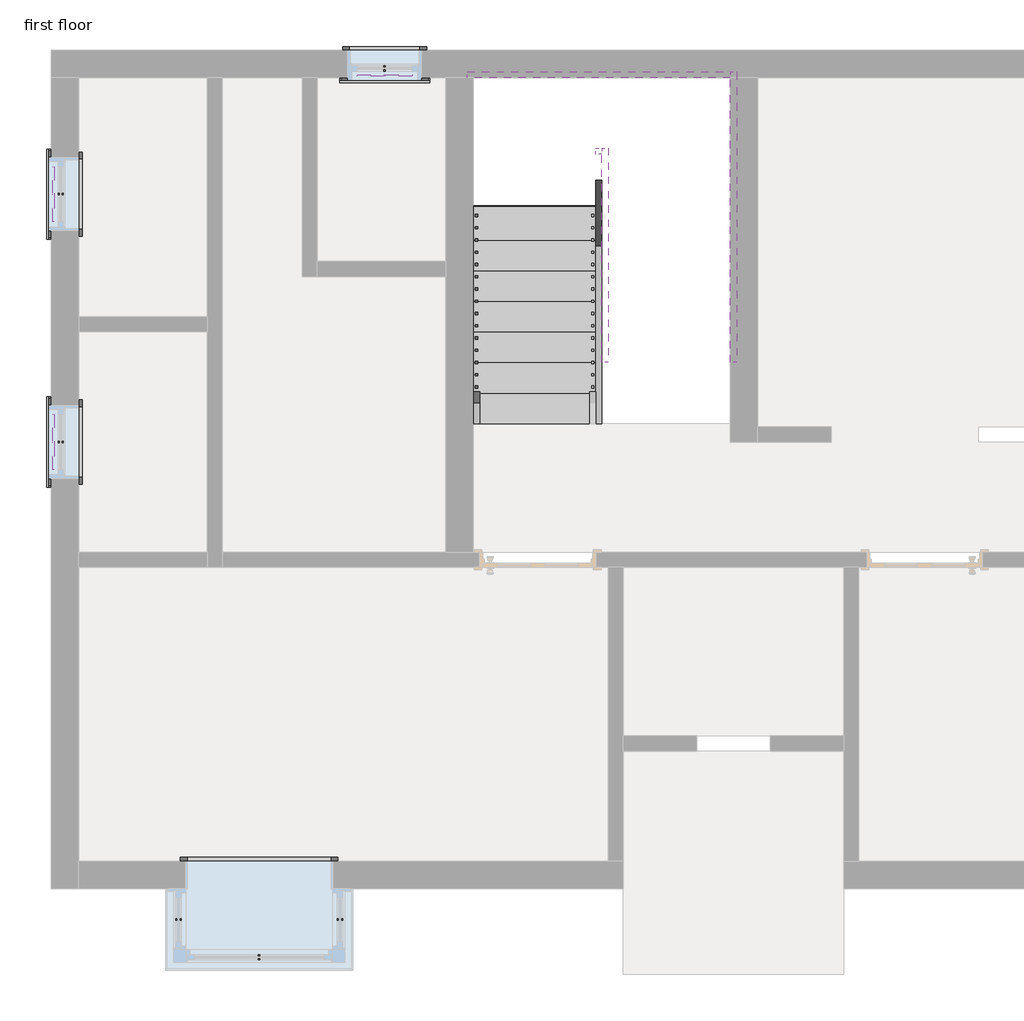
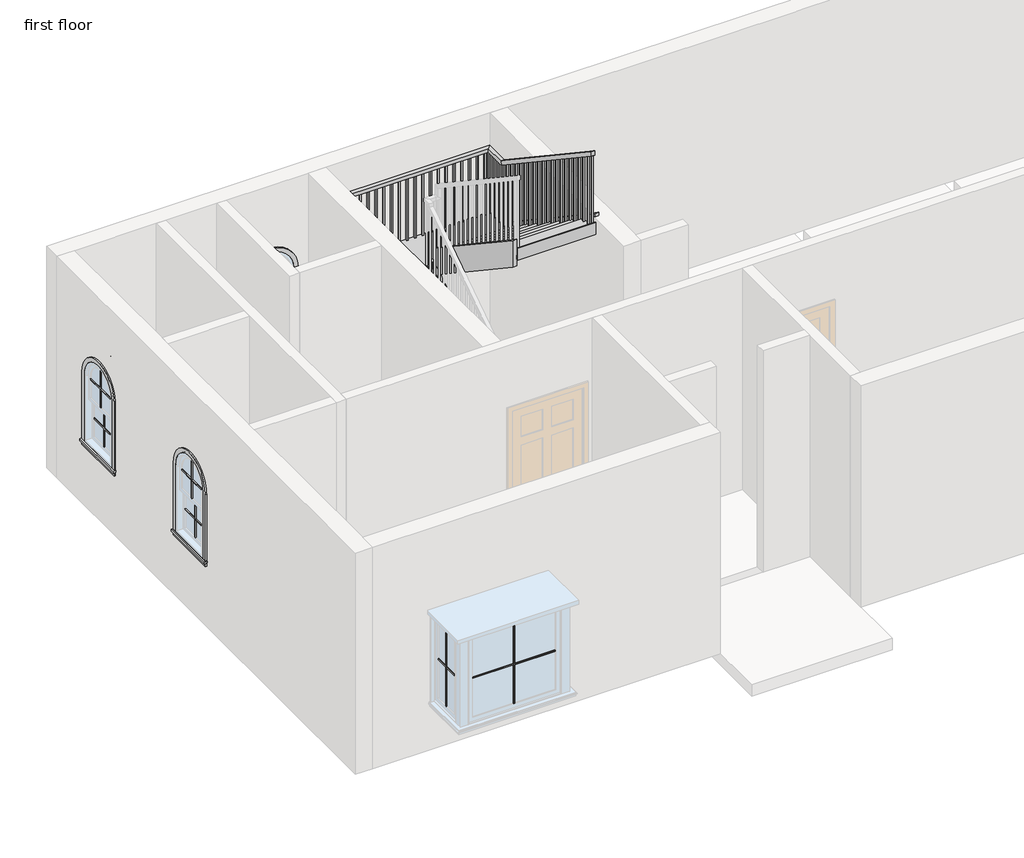
# One storey, part 3 of 3: 16 proxies, 6 members, 1 railing, 1 stair flight.
"""IFC4 building model written with IfcOpenShell, lengths in millimetres."""

from ifc_helpers import new_model, si_unit, frame, origin, place, context, project, spatial, polyline, outline, extrude, faceted_brep, transform, mapped, element, save
from components import muntin_pattern_2x2_muntin_pattern_2x2_3440c8d2, muntin_pattern_2x2_muntin_pattern_2x2_8235f178, muntin_pattern_2x2_muntin_pattern_2x2_f03ab90d, trim_window_exterior_arch_hung_with_sill_ae9dfc94, trim_window_interior_arch_hung_picture_frame_76300bdb, trim_window_interior_flat_picture_frame_ace0ae79, stair_flight_5c93b7ad

model = new_model("IFC4")

# Units and contexts
model_context = context("Model", 3, world=origin())
ifc_project = project(units=[si_unit("LENGTHUNIT", "METRE", prefix="MILLI")], contexts=[model_context])

# Site, building, storey
site = spatial("IfcSite", under=ifc_project)
building = spatial("IfcBuilding", under=site)
storey = spatial("IfcBuildingStorey", under=building, Name="first floor", Elevation=3352.8)

# Proxies
placement = place(None, origin())
muntin_pattern_2x2_muntin_pattern_2x2_shape = muntin_pattern_2x2_muntin_pattern_2x2_3440c8d2(model_context)
element("IfcBuildingElementProxy", 1, Name="Muntin Pattern_2x2 : Muntin Pattern_2x2", ObjectType="Muntin Pattern_2x2 : Muntin Pattern_2x2", at=placement, inside=storey, context=model_context, shape_type="MappedRepresentation", body=[
    mapped(muntin_pattern_2x2_muntin_pattern_2x2_shape, transform((-13144.1422301, -1499.4302427, 4899.025), x_axis=(0.0, 1.0, 0.0), y_axis=(-1.0, 0.0, 0.0), z_axis=(0.0, 0.0, 1.0))),
])
element("IfcBuildingElementProxy", 2, Name="Muntin Pattern_2x2 : Muntin Pattern_2x2", ObjectType="Muntin Pattern_2x2 : Muntin Pattern_2x2", at=placement, inside=storey, context=model_context, shape_type="MappedRepresentation", body=[
    mapped(muntin_pattern_2x2_muntin_pattern_2x2_shape, transform((-13099.6922301, -1499.4302427, 4343.4), x_axis=(0.0, 1.0, 0.0), y_axis=(-1.0, 0.0, 0.0), z_axis=(0.0, 0.0, 1.0))),
])
element("IfcBuildingElementProxy", 3, Name="Muntin Pattern_2x2 : Muntin Pattern_2x2", ObjectType="Muntin Pattern_2x2 : Muntin Pattern_2x2", at=placement, inside=storey, context=model_context, shape_type="MappedRepresentation", body=[
    mapped(muntin_pattern_2x2_muntin_pattern_2x2_shape, transform((-13144.1422301, -3556.8302427, 4899.025), x_axis=(0.0, 1.0, 0.0), y_axis=(-1.0, 0.0, 0.0), z_axis=(0.0, 0.0, 1.0))),
])
element("IfcBuildingElementProxy", 4, Name="Muntin Pattern_2x2 : Muntin Pattern_2x2", ObjectType="Muntin Pattern_2x2 : Muntin Pattern_2x2", at=placement, inside=storey, context=model_context, shape_type="MappedRepresentation", body=[
    mapped(muntin_pattern_2x2_muntin_pattern_2x2_shape, transform((-13099.6922301, -3556.8302427, 4343.4), x_axis=(0.0, 1.0, 0.0), y_axis=(-1.0, 0.0, 0.0), z_axis=(0.0, 0.0, 1.0))),
])
element("IfcBuildingElementProxy", 5, Name="Muntin Pattern_2x2 : Muntin Pattern_2x2", ObjectType="Muntin Pattern_2x2 : Muntin Pattern_2x2", at=placement, inside=storey, context=model_context, shape_type="MappedRepresentation", body=[
    mapped(muntin_pattern_2x2_muntin_pattern_2x2_shape, transform((-10410.4672301, -499.3052427, 4899.025), x_axis=(-1.0, 0.0, 0.0), y_axis=(0.0, -1.0, 0.0), z_axis=(0.0, 0.0, 1.0))),
])
element("IfcBuildingElementProxy", 6, Name="Muntin Pattern_2x2 : Muntin Pattern_2x2", ObjectType="Muntin Pattern_2x2 : Muntin Pattern_2x2", at=placement, inside=storey, context=model_context, shape_type="MappedRepresentation", body=[
    mapped(muntin_pattern_2x2_muntin_pattern_2x2_shape, transform((-10410.4672301, -454.8552427, 4343.4), x_axis=(-1.0, 0.0, 0.0), y_axis=(0.0, -1.0, 0.0), z_axis=(0.0, 0.0, 1.0))),
])
muntin_pattern_2x2_muntin_pattern_2x2_2_shape = muntin_pattern_2x2_muntin_pattern_2x2_8235f178(model_context)
element("IfcBuildingElementProxy", 7, Name="Muntin Pattern_2x2 : Muntin Pattern_2x2", ObjectType="Muntin Pattern_2x2 : Muntin Pattern_2x2", at=placement, inside=storey, context=model_context, shape_type="MappedRepresentation", body=[
    mapped(muntin_pattern_2x2_muntin_pattern_2x2_2_shape, transform((-11451.8672301, -7833.5552427, 4083.05), x_axis=(-1.0, 0.0, 0.0), y_axis=(0.0, -1.0, 0.0), z_axis=(0.0, 0.0, 1.0))),
])
muntin_pattern_2x2_muntin_pattern_2x2_3_shape = muntin_pattern_2x2_muntin_pattern_2x2_f03ab90d(model_context)
element("IfcBuildingElementProxy", 8, Name="Muntin Pattern_2x2 : Muntin Pattern_2x2", ObjectType="Muntin Pattern_2x2 : Muntin Pattern_2x2", at=placement, inside=storey, context=model_context, shape_type="MappedRepresentation", body=[
    mapped(muntin_pattern_2x2_muntin_pattern_2x2_3_shape, transform((-10781.9422301, -7519.2302427, 4083.05), x_axis=(0.0, 1.0, 0.0), y_axis=(-1.0, 0.0, 0.0), z_axis=(0.0, 0.0, 1.0))),
])
element("IfcBuildingElementProxy", 9, Name="Muntin Pattern_2x2 : Muntin Pattern_2x2", ObjectType="Muntin Pattern_2x2 : Muntin Pattern_2x2", at=placement, inside=storey, context=model_context, shape_type="MappedRepresentation", body=[
    mapped(muntin_pattern_2x2_muntin_pattern_2x2_3_shape, transform((-12121.7922301, -7519.2302427, 4083.05), x_axis=(0.0, -1.0, 0.0), y_axis=(1.0, 0.0, 0.0), z_axis=(0.0, 0.0, 1.0))),
])
trim_window_exterior_arch_hung_with_sill_shape = trim_window_exterior_arch_hung_with_sill_ae9dfc94(model_context)
element("IfcBuildingElementProxy", 10, Name="Trim-Window-Exterior-Arch-Hung : with Sill", ObjectType="Trim-Window-Exterior-Arch-Hung : with Sill", at=placement, inside=storey, context=model_context, shape_type="MappedRepresentation", body=[
    mapped(trim_window_exterior_arch_hung_with_sill_shape, transform((-13179.0672301, -1499.4302427, 5486.4), x_axis=(0.0, -1.0, 0.0), y_axis=(0.0, 0.0, 1.0), z_axis=(-1.0, 0.0, 0.0))),
])
element("IfcBuildingElementProxy", 11, Name="Trim-Window-Exterior-Arch-Hung : with Sill", ObjectType="Trim-Window-Exterior-Arch-Hung : with Sill", at=placement, inside=storey, context=model_context, shape_type="MappedRepresentation", body=[
    mapped(trim_window_exterior_arch_hung_with_sill_shape, transform((-13179.0672301, -3556.8302427, 5486.4), x_axis=(0.0, -1.0, 0.0), y_axis=(0.0, 0.0, 1.0), z_axis=(-1.0, 0.0, 0.0))),
])
element("IfcBuildingElementProxy", 12, Name="Trim-Window-Exterior-Arch-Hung : with Sill", ObjectType="Trim-Window-Exterior-Arch-Hung : with Sill", at=placement, inside=storey, context=model_context, shape_type="MappedRepresentation", body=[
    mapped(trim_window_exterior_arch_hung_with_sill_shape, transform((-10410.4672301, -534.2302427, 5486.4), x_axis=(1.0, 0.0, 0.0), y_axis=(0.0, 0.0, 1.0), z_axis=(0.0, -1.0, 0.0))),
])
trim_window_interior_arch_hung_picture_frame_shape = trim_window_interior_arch_hung_picture_frame_76300bdb(model_context)
element("IfcBuildingElementProxy", 13, Name="Trim-Window-Interior-Arch-Hung : Picture Frame", ObjectType="Trim-Window-Interior-Arch-Hung : Picture Frame", at=placement, inside=storey, context=model_context, shape_type="MappedRepresentation", body=[
    mapped(trim_window_interior_arch_hung_picture_frame_shape, transform((-12950.4672301, -1499.4302427, 5486.4), x_axis=(0.0, 1.0, 0.0), y_axis=(0.0, 0.0, 1.0), z_axis=(1.0, 0.0, 0.0))),
])
element("IfcBuildingElementProxy", 14, Name="Trim-Window-Interior-Arch-Hung : Picture Frame", ObjectType="Trim-Window-Interior-Arch-Hung : Picture Frame", at=placement, inside=storey, context=model_context, shape_type="MappedRepresentation", body=[
    mapped(trim_window_interior_arch_hung_picture_frame_shape, transform((-12950.4672301, -3556.8302427, 5486.4), x_axis=(0.0, 1.0, 0.0), y_axis=(0.0, 0.0, 1.0), z_axis=(1.0, 0.0, 0.0))),
])
element("IfcBuildingElementProxy", 15, Name="Trim-Window-Interior-Arch-Hung : Picture Frame", ObjectType="Trim-Window-Interior-Arch-Hung : Picture Frame", at=placement, inside=storey, context=model_context, shape_type="MappedRepresentation", body=[
    mapped(trim_window_interior_arch_hung_picture_frame_shape, transform((-10410.4672301, -305.6302427, 5486.4), x_axis=(-1.0, 0.0, 0.0), y_axis=(0.0, 0.0, 1.0), z_axis=(0.0, 1.0, 0.0))),
])
trim_window_interior_flat_picture_frame_shape = trim_window_interior_flat_picture_frame_ace0ae79(model_context)
element("IfcBuildingElementProxy", 16, Name="Trim-Window-Interior-Flat : Picture Frame", ObjectType="Trim-Window-Interior-Flat : Picture Frame", at=placement, inside=storey, context=model_context, shape_type="MappedRepresentation", body=[
    mapped(trim_window_interior_flat_picture_frame_shape, transform((-11451.8672301, -7036.6302427, 5232.4), x_axis=(-1.0, 0.0, 0.0), y_axis=(0.0, 0.0, 1.0), z_axis=(0.0, 1.0, 0.0))),
])

# Members
element("IfcMember", 17, ObjectType="Stringer - 2\" Width", at=placement, inside=storey, context=model_context, shape_type="SweptSolid", body=[
    extrude(outline(polyline([(-3404.4302427, 3352.8), (-3404.4302427, 3570.8398409), (-1077.1900041, 5122.3333333), (-534.2302427, 5122.3333333), (-534.2302427, 5117.982498), (-3182.0039897, 3352.8), (-3404.4302427, 3352.8)])), frame((-9724.6672301, 0.0, 0.0), z_axis=(1.0, 0.0, 0.0), x_axis=(0.0, 1.0, 0.0)), (0.0, 0.0, 1.0), 50.8),
])
element("IfcMember", 18, ObjectType="Stringer - 2\" Width", at=placement, inside=storey, context=model_context, shape_type="SweptSolid", body=[
    extrude(outline(polyline([(-9724.6672301, -534.2302427), (-9724.6672301, -483.4302427), (-7540.2672301, -483.4302427), (-7540.2672301, -534.2302427), (-9724.6672301, -534.2302427)])), frame((0.0, 0.0, 4817.5333333), z_axis=(0.0, 0.0, 1.0), x_axis=(1.0, 0.0, 0.0)), (0.0, 0.0, 1.0), 304.8),
])
element("IfcMember", 19, ObjectType="Stringer - 2\" Width", at=placement, inside=storey, context=model_context, shape_type="SweptSolid", body=[
    extrude(outline(polyline([(-483.4302427, 4840.8398409), (-483.4302427, 4817.5333333), (-997.9564957, 4817.5333333), (-2896.4302427, 6083.182498), (-2896.4302427, 6449.5065076), (-483.4302427, 4840.8398409)])), frame((-7540.2672301, 0.0, 0.0), z_axis=(1.0, 0.0, 0.0), x_axis=(0.0, 1.0, 0.0)), (0.0, 0.0, 1.0), 50.8),
])
element("IfcMember", 20, ObjectType="Stringer - 2\" Width", at=placement, inside=storey, context=model_context, shape_type="SweptSolid", body=[
    extrude(outline(polyline([(-3404.4302427, 3352.8), (-3404.4302427, 3570.8398409), (-1169.2302427, 5060.9731743), (-1169.2302427, 4694.6491647), (-3182.0039897, 3352.8), (-3404.4302427, 3352.8)])), frame((-8657.8672301, 0.0, 0.0), z_axis=(1.0, 0.0, 0.0), x_axis=(0.0, 1.0, 0.0)), (0.0, 0.0, 1.0), 50.8),
])
element("IfcMember", 21, ObjectType="Stringer - 2\" Width", at=placement, inside=storey, context=model_context, shape_type="SweptSolid", body=[
    extrude(outline(polyline([(-8657.8672301, -1169.2302427), (-8657.8672301, -1118.4302427), (-8607.0672301, -1118.4302427), (-8607.0672301, -1169.2302427), (-8657.8672301, -1169.2302427)])), frame((0.0, 0.0, 4817.5333333), z_axis=(0.0, 0.0, 1.0), x_axis=(1.0, 0.0, 0.0)), (0.0, 0.0, 1.0), 304.8),
])
element("IfcMember", 22, ObjectType="Stringer - 2\" Width", at=placement, inside=storey, context=model_context, shape_type="SweptSolid", body=[
    extrude(outline(polyline([(-1118.4302427, 5264.1731743), (-1118.4302427, 4897.8491647), (-2896.4302427, 6083.182498), (-2896.4302427, 6449.5065076), (-1118.4302427, 5264.1731743)])), frame((-8607.0672301, 0.0, 0.0), z_axis=(1.0, 0.0, 0.0), x_axis=(0.0, 1.0, 0.0)), (0.0, 0.0, 1.0), 50.8),
])

# Railing
element("IfcRailing", 23, ObjectType="Handrail - Rectangular", at=placement, inside=storey, context=model_context, shape_type="SolidModel", body=[
    faceted_brep([(-9673.8672301, -3404.4302427, 4436.5333333), (-9673.8672301, -3404.4302427, 4375.4793317), (-9623.0672301, -3404.4302427, 4375.4793317), (-9623.0672301, -3404.4302427, 4436.5333333), (-9673.8672301, -1118.4302427, 5960.5333333), (-9673.8672301, -1103.0492403, 5909.7333333), (-9623.0672301, -1103.0492403, 5909.7333333), (-9623.0672301, -1118.4302427, 5960.5333333), (-9673.8672301, -534.2302427, 5960.5333333), (-9673.8672301, -534.2302427, 5909.7333333), (-9623.0672301, -585.0302427, 5909.7333333), (-9623.0672301, -585.0302427, 5960.5333333), (-7540.2672301, -534.2302427, 5960.5333333), (-7540.2672301, -534.2302427, 5909.7333333), (-7591.0672301, -585.0302427, 5909.7333333), (-7591.0672301, -585.0302427, 5960.5333333), (-7540.2672301, -864.4302427, 5960.5333333), (-7540.2672301, -879.8112451, 5909.7333333), (-7591.0672301, -879.8112451, 5909.7333333), (-7591.0672301, -864.4302427, 5960.5333333), (-7540.2672301, -2896.4302427, 7315.2), (-7591.0672301, -2896.4302427, 7315.2), (-7591.0672301, -2896.4302427, 7254.1459984), (-7540.2672301, -2896.4302427, 7254.1459984)], [[[0, 1, 2, 3]], [[1, 0, 4, 5]], [[2, 1, 5, 6]], [[3, 2, 6, 7]], [[0, 3, 7, 4]], [[5, 4, 8, 9]], [[6, 5, 9, 10]], [[7, 6, 10, 11]], [[4, 7, 11, 8]], [[9, 8, 12, 13]], [[10, 9, 13, 14]], [[11, 10, 14, 15]], [[8, 11, 15, 12]], [[13, 12, 16, 17]], [[14, 13, 17, 18]], [[15, 14, 18, 19]], [[12, 15, 19, 16]], [[20, 21, 22, 23]], [[17, 16, 20, 23]], [[18, 17, 23, 22]], [[19, 18, 22, 21]], [[16, 19, 21, 20]]]),
    extrude(outline(polyline([(-2785.3052427, 7180.0626651), (-2785.3052427, 6231.4666667), (-2804.3552427, 6231.4666667), (-2804.3552427, 7192.7626651), (-2785.3052427, 7180.0626651)])), frame((-7575.1922301, 0.0, 0.0), z_axis=(1.0, 0.0, 0.0), x_axis=(0.0, 1.0, 0.0)), (0.0, 0.0, 1.0), 19.05),
    extrude(outline(polyline([(-2683.7052427, 7112.3293317), (-2683.7052427, 6231.4666667), (-2702.7552427, 6231.4666667), (-2702.7552427, 7125.0293317), (-2683.7052427, 7112.3293317)])), frame((-7575.1922301, 0.0, 0.0), z_axis=(1.0, 0.0, 0.0), x_axis=(0.0, 1.0, 0.0)), (0.0, 0.0, 1.0), 19.05),
    extrude(outline(polyline([(-2582.1052427, 7044.5959984), (-2582.1052427, 6062.1333333), (-2601.1552427, 6062.1333333), (-2601.1552427, 7057.2959984), (-2582.1052427, 7044.5959984)])), frame((-7575.1922301, 0.0, 0.0), z_axis=(1.0, 0.0, 0.0), x_axis=(0.0, 1.0, 0.0)), (0.0, 0.0, 1.0), 19.05),
    extrude(outline(polyline([(-2480.5052427, 6976.8626651), (-2480.5052427, 6062.1333333), (-2499.5552427, 6062.1333333), (-2499.5552427, 6989.5626651), (-2480.5052427, 6976.8626651)])), frame((-7575.1922301, 0.0, 0.0), z_axis=(1.0, 0.0, 0.0), x_axis=(0.0, 1.0, 0.0)), (0.0, 0.0, 1.0), 19.05),
    extrude(outline(polyline([(-2378.9052427, 6909.1293317), (-2378.9052427, 6062.1333333), (-2397.9552427, 6062.1333333), (-2397.9552427, 6921.8293317), (-2378.9052427, 6909.1293317)])), frame((-7575.1922301, 0.0, 0.0), z_axis=(1.0, 0.0, 0.0), x_axis=(0.0, 1.0, 0.0)), (0.0, 0.0, 1.0), 19.05),
    extrude(outline(polyline([(-2277.3052427, 6841.3959984), (-2277.3052427, 5892.8), (-2296.3552427, 5892.8), (-2296.3552427, 6854.0959984), (-2277.3052427, 6841.3959984)])), frame((-7575.1922301, 0.0, 0.0), z_axis=(1.0, 0.0, 0.0), x_axis=(0.0, 1.0, 0.0)), (0.0, 0.0, 1.0), 19.05),
    extrude(outline(polyline([(-2175.7052427, 6773.6626651), (-2175.7052427, 5892.8), (-2194.7552427, 5892.8), (-2194.7552427, 6786.3626651), (-2175.7052427, 6773.6626651)])), frame((-7575.1922301, 0.0, 0.0), z_axis=(1.0, 0.0, 0.0), x_axis=(0.0, 1.0, 0.0)), (0.0, 0.0, 1.0), 19.05),
    extrude(outline(polyline([(-2074.1052427, 6705.9293317), (-2074.1052427, 5723.4666667), (-2093.1552427, 5723.4666667), (-2093.1552427, 6718.6293317), (-2074.1052427, 6705.9293317)])), frame((-7575.1922301, 0.0, 0.0), z_axis=(1.0, 0.0, 0.0), x_axis=(0.0, 1.0, 0.0)), (0.0, 0.0, 1.0), 19.05),
    extrude(outline(polyline([(-1972.5052427, 6638.1959984), (-1972.5052427, 5723.4666667), (-1991.5552427, 5723.4666667), (-1991.5552427, 6650.8959984), (-1972.5052427, 6638.1959984)])), frame((-7575.1922301, 0.0, 0.0), z_axis=(1.0, 0.0, 0.0), x_axis=(0.0, 1.0, 0.0)), (0.0, 0.0, 1.0), 19.05),
    extrude(outline(polyline([(-1870.9052427, 6570.4626651), (-1870.9052427, 5723.4666667), (-1889.9552427, 5723.4666667), (-1889.9552427, 6583.1626651), (-1870.9052427, 6570.4626651)])), frame((-7575.1922301, 0.0, 0.0), z_axis=(1.0, 0.0, 0.0), x_axis=(0.0, 1.0, 0.0)), (0.0, 0.0, 1.0), 19.05),
    extrude(outline(polyline([(-1769.3052427, 6502.7293317), (-1769.3052427, 5554.1333333), (-1788.3552427, 5554.1333333), (-1788.3552427, 6515.4293317), (-1769.3052427, 6502.7293317)])), frame((-7575.1922301, 0.0, 0.0), z_axis=(1.0, 0.0, 0.0), x_axis=(0.0, 1.0, 0.0)), (0.0, 0.0, 1.0), 19.05),
    extrude(outline(polyline([(-1667.7052427, 6434.9959984), (-1667.7052427, 5554.1333333), (-1686.7552427, 5554.1333333), (-1686.7552427, 6447.6959984), (-1667.7052427, 6434.9959984)])), frame((-7575.1922301, 0.0, 0.0), z_axis=(1.0, 0.0, 0.0), x_axis=(0.0, 1.0, 0.0)), (0.0, 0.0, 1.0), 19.05),
    extrude(outline(polyline([(-1566.1052427, 6367.2626651), (-1566.1052427, 5384.8), (-1585.1552427, 5384.8), (-1585.1552427, 6379.9626651), (-1566.1052427, 6367.2626651)])), frame((-7575.1922301, 0.0, 0.0), z_axis=(1.0, 0.0, 0.0), x_axis=(0.0, 1.0, 0.0)), (0.0, 0.0, 1.0), 19.05),
    extrude(outline(polyline([(-1464.5052427, 6299.5293317), (-1464.5052427, 5384.8), (-1483.5552427, 5384.8), (-1483.5552427, 6312.2293317), (-1464.5052427, 6299.5293317)])), frame((-7575.1922301, 0.0, 0.0), z_axis=(1.0, 0.0, 0.0), x_axis=(0.0, 1.0, 0.0)), (0.0, 0.0, 1.0), 19.05),
    extrude(outline(polyline([(-1362.9052427, 6231.7959984), (-1362.9052427, 5384.8), (-1381.9552427, 5384.8), (-1381.9552427, 6244.4959984), (-1362.9052427, 6231.7959984)])), frame((-7575.1922301, 0.0, 0.0), z_axis=(1.0, 0.0, 0.0), x_axis=(0.0, 1.0, 0.0)), (0.0, 0.0, 1.0), 19.05),
    extrude(outline(polyline([(-1261.3052427, 6164.0626651), (-1261.3052427, 5215.4666667), (-1280.3552427, 5215.4666667), (-1280.3552427, 6176.7626651), (-1261.3052427, 6164.0626651)])), frame((-7575.1922301, 0.0, 0.0), z_axis=(1.0, 0.0, 0.0), x_axis=(0.0, 1.0, 0.0)), (0.0, 0.0, 1.0), 19.05),
    extrude(outline(polyline([(-1159.7052427, 6096.3293317), (-1159.7052427, 5215.4666667), (-1178.7552427, 5215.4666667), (-1178.7552427, 6109.0293317), (-1159.7052427, 6096.3293317)])), frame((-7575.1922301, 0.0, 0.0), z_axis=(1.0, 0.0, 0.0), x_axis=(0.0, 1.0, 0.0)), (0.0, 0.0, 1.0), 19.05),
    extrude(outline(polyline([(-1058.1052427, 6028.5959984), (-1058.1052427, 5046.1333333), (-1077.1552427, 5046.1333333), (-1077.1552427, 6041.2959984), (-1058.1052427, 6028.5959984)])), frame((-7575.1922301, 0.0, 0.0), z_axis=(1.0, 0.0, 0.0), x_axis=(0.0, 1.0, 0.0)), (0.0, 0.0, 1.0), 19.05),
    extrude(outline(polyline([(-956.5052427, 5960.8626651), (-956.5052427, 5046.1333333), (-975.5552427, 5046.1333333), (-975.5552427, 5973.5626651), (-956.5052427, 5960.8626651)])), frame((-7575.1922301, 0.0, 0.0), z_axis=(1.0, 0.0, 0.0), x_axis=(0.0, 1.0, 0.0)), (0.0, 0.0, 1.0), 19.05),
    extrude(outline(polyline([(-7556.1422301, -854.9052427), (-7556.1422301, -873.9552427), (-7575.1922301, -873.9552427), (-7575.1922301, -854.9052427), (-7556.1422301, -854.9052427)])), frame((0.0, 0.0, 5046.1333333), z_axis=(0.0, 0.0, 1.0), x_axis=(1.0, 0.0, 0.0)), (0.0, 0.0, 1.0), 863.6),
    extrude(outline(polyline([(-7556.1422301, -753.3052427), (-7556.1422301, -772.3552427), (-7575.1922301, -772.3552427), (-7575.1922301, -753.3052427), (-7556.1422301, -753.3052427)])), frame((0.0, 0.0, 5046.1333333), z_axis=(0.0, 0.0, 1.0), x_axis=(1.0, 0.0, 0.0)), (0.0, 0.0, 1.0), 863.6),
    extrude(outline(polyline([(-7556.1422301, -651.7052427), (-7556.1422301, -670.7552427), (-7575.1922301, -670.7552427), (-7575.1922301, -651.7052427), (-7556.1422301, -651.7052427)])), frame((0.0, 0.0, 5046.1333333), z_axis=(0.0, 0.0, 1.0), x_axis=(1.0, 0.0, 0.0)), (0.0, 0.0, 1.0), 863.6),
    extrude(outline(polyline([(-7625.9922301, -550.1052427), (-7606.9422301, -550.1052427), (-7606.9422301, -569.1552427), (-7625.9922301, -569.1552427), (-7625.9922301, -550.1052427)])), frame((0.0, 0.0, 5046.1333333), z_axis=(0.0, 0.0, 1.0), x_axis=(1.0, 0.0, 0.0)), (0.0, 0.0, 1.0), 863.6),
    extrude(outline(polyline([(-7727.5922301, -550.1052427), (-7708.5422301, -550.1052427), (-7708.5422301, -569.1552427), (-7727.5922301, -569.1552427), (-7727.5922301, -550.1052427)])), frame((0.0, 0.0, 5046.1333333), z_axis=(0.0, 0.0, 1.0), x_axis=(1.0, 0.0, 0.0)), (0.0, 0.0, 1.0), 863.6),
    extrude(outline(polyline([(-7829.1922301, -550.1052427), (-7810.1422301, -550.1052427), (-7810.1422301, -569.1552427), (-7829.1922301, -569.1552427), (-7829.1922301, -550.1052427)])), frame((0.0, 0.0, 5046.1333333), z_axis=(0.0, 0.0, 1.0), x_axis=(1.0, 0.0, 0.0)), (0.0, 0.0, 1.0), 863.6),
    extrude(outline(polyline([(-7930.7922301, -550.1052427), (-7911.7422301, -550.1052427), (-7911.7422301, -569.1552427), (-7930.7922301, -569.1552427), (-7930.7922301, -550.1052427)])), frame((0.0, 0.0, 5046.1333333), z_axis=(0.0, 0.0, 1.0), x_axis=(1.0, 0.0, 0.0)), (0.0, 0.0, 1.0), 863.6),
    extrude(outline(polyline([(-8032.3922301, -550.1052427), (-8013.3422301, -550.1052427), (-8013.3422301, -569.1552427), (-8032.3922301, -569.1552427), (-8032.3922301, -550.1052427)])), frame((0.0, 0.0, 5046.1333333), z_axis=(0.0, 0.0, 1.0), x_axis=(1.0, 0.0, 0.0)), (0.0, 0.0, 1.0), 863.6),
    extrude(outline(polyline([(-8133.9922301, -550.1052427), (-8114.9422301, -550.1052427), (-8114.9422301, -569.1552427), (-8133.9922301, -569.1552427), (-8133.9922301, -550.1052427)])), frame((0.0, 0.0, 5046.1333333), z_axis=(0.0, 0.0, 1.0), x_axis=(1.0, 0.0, 0.0)), (0.0, 0.0, 1.0), 863.6),
    extrude(outline(polyline([(-8235.5922301, -550.1052427), (-8216.5422301, -550.1052427), (-8216.5422301, -569.1552427), (-8235.5922301, -569.1552427), (-8235.5922301, -550.1052427)])), frame((0.0, 0.0, 5046.1333333), z_axis=(0.0, 0.0, 1.0), x_axis=(1.0, 0.0, 0.0)), (0.0, 0.0, 1.0), 863.6),
    extrude(outline(polyline([(-8337.1922301, -550.1052427), (-8318.1422301, -550.1052427), (-8318.1422301, -569.1552427), (-8337.1922301, -569.1552427), (-8337.1922301, -550.1052427)])), frame((0.0, 0.0, 5046.1333333), z_axis=(0.0, 0.0, 1.0), x_axis=(1.0, 0.0, 0.0)), (0.0, 0.0, 1.0), 863.6),
    extrude(outline(polyline([(-8438.7922301, -550.1052427), (-8419.7422301, -550.1052427), (-8419.7422301, -569.1552427), (-8438.7922301, -569.1552427), (-8438.7922301, -550.1052427)])), frame((0.0, 0.0, 5046.1333333), z_axis=(0.0, 0.0, 1.0), x_axis=(1.0, 0.0, 0.0)), (0.0, 0.0, 1.0), 863.6),
    extrude(outline(polyline([(-8540.3922301, -550.1052427), (-8521.3422301, -550.1052427), (-8521.3422301, -569.1552427), (-8540.3922301, -569.1552427), (-8540.3922301, -550.1052427)])), frame((0.0, 0.0, 5046.1333333), z_axis=(0.0, 0.0, 1.0), x_axis=(1.0, 0.0, 0.0)), (0.0, 0.0, 1.0), 863.6),
    extrude(outline(polyline([(-8641.9922301, -550.1052427), (-8622.9422301, -550.1052427), (-8622.9422301, -569.1552427), (-8641.9922301, -569.1552427), (-8641.9922301, -550.1052427)])), frame((0.0, 0.0, 5046.1333333), z_axis=(0.0, 0.0, 1.0), x_axis=(1.0, 0.0, 0.0)), (0.0, 0.0, 1.0), 863.6),
    extrude(outline(polyline([(-8743.5922301, -550.1052427), (-8724.5422301, -550.1052427), (-8724.5422301, -569.1552427), (-8743.5922301, -569.1552427), (-8743.5922301, -550.1052427)])), frame((0.0, 0.0, 5046.1333333), z_axis=(0.0, 0.0, 1.0), x_axis=(1.0, 0.0, 0.0)), (0.0, 0.0, 1.0), 863.6),
    extrude(outline(polyline([(-8845.1922301, -550.1052427), (-8826.1422301, -550.1052427), (-8826.1422301, -569.1552427), (-8845.1922301, -569.1552427), (-8845.1922301, -550.1052427)])), frame((0.0, 0.0, 5046.1333333), z_axis=(0.0, 0.0, 1.0), x_axis=(1.0, 0.0, 0.0)), (0.0, 0.0, 1.0), 863.6),
    extrude(outline(polyline([(-8946.7922301, -550.1052427), (-8927.7422301, -550.1052427), (-8927.7422301, -569.1552427), (-8946.7922301, -569.1552427), (-8946.7922301, -550.1052427)])), frame((0.0, 0.0, 5046.1333333), z_axis=(0.0, 0.0, 1.0), x_axis=(1.0, 0.0, 0.0)), (0.0, 0.0, 1.0), 863.6),
    extrude(outline(polyline([(-9048.3922301, -550.1052427), (-9029.3422301, -550.1052427), (-9029.3422301, -569.1552427), (-9048.3922301, -569.1552427), (-9048.3922301, -550.1052427)])), frame((0.0, 0.0, 5046.1333333), z_axis=(0.0, 0.0, 1.0), x_axis=(1.0, 0.0, 0.0)), (0.0, 0.0, 1.0), 863.6),
    extrude(outline(polyline([(-9149.9922301, -550.1052427), (-9130.9422301, -550.1052427), (-9130.9422301, -569.1552427), (-9149.9922301, -569.1552427), (-9149.9922301, -550.1052427)])), frame((0.0, 0.0, 5046.1333333), z_axis=(0.0, 0.0, 1.0), x_axis=(1.0, 0.0, 0.0)), (0.0, 0.0, 1.0), 863.6),
    extrude(outline(polyline([(-9251.5922301, -550.1052427), (-9232.5422301, -550.1052427), (-9232.5422301, -569.1552427), (-9251.5922301, -569.1552427), (-9251.5922301, -550.1052427)])), frame((0.0, 0.0, 5046.1333333), z_axis=(0.0, 0.0, 1.0), x_axis=(1.0, 0.0, 0.0)), (0.0, 0.0, 1.0), 863.6),
    extrude(outline(polyline([(-9353.1922301, -550.1052427), (-9334.1422301, -550.1052427), (-9334.1422301, -569.1552427), (-9353.1922301, -569.1552427), (-9353.1922301, -550.1052427)])), frame((0.0, 0.0, 5046.1333333), z_axis=(0.0, 0.0, 1.0), x_axis=(1.0, 0.0, 0.0)), (0.0, 0.0, 1.0), 863.6),
    extrude(outline(polyline([(-9454.7922301, -550.1052427), (-9435.7422301, -550.1052427), (-9435.7422301, -569.1552427), (-9454.7922301, -569.1552427), (-9454.7922301, -550.1052427)])), frame((0.0, 0.0, 5046.1333333), z_axis=(0.0, 0.0, 1.0), x_axis=(1.0, 0.0, 0.0)), (0.0, 0.0, 1.0), 863.6),
    extrude(outline(polyline([(-9556.3922301, -550.1052427), (-9537.3422301, -550.1052427), (-9537.3422301, -569.1552427), (-9556.3922301, -569.1552427), (-9556.3922301, -550.1052427)])), frame((0.0, 0.0, 5046.1333333), z_axis=(0.0, 0.0, 1.0), x_axis=(1.0, 0.0, 0.0)), (0.0, 0.0, 1.0), 863.6),
    extrude(outline(polyline([(-9657.9922301, -670.7552427), (-9657.9922301, -651.7052427), (-9638.9422301, -651.7052427), (-9638.9422301, -670.7552427), (-9657.9922301, -670.7552427)])), frame((0.0, 0.0, 5046.1333333), z_axis=(0.0, 0.0, 1.0), x_axis=(1.0, 0.0, 0.0)), (0.0, 0.0, 1.0), 863.6),
    extrude(outline(polyline([(-9657.9922301, -772.3552427), (-9657.9922301, -753.3052427), (-9638.9422301, -753.3052427), (-9638.9422301, -772.3552427), (-9657.9922301, -772.3552427)])), frame((0.0, 0.0, 5046.1333333), z_axis=(0.0, 0.0, 1.0), x_axis=(1.0, 0.0, 0.0)), (0.0, 0.0, 1.0), 863.6),
    extrude(outline(polyline([(-9657.9922301, -873.9552427), (-9657.9922301, -854.9052427), (-9638.9422301, -854.9052427), (-9638.9422301, -873.9552427), (-9657.9922301, -873.9552427)])), frame((0.0, 0.0, 5046.1333333), z_axis=(0.0, 0.0, 1.0), x_axis=(1.0, 0.0, 0.0)), (0.0, 0.0, 1.0), 863.6),
    extrude(outline(polyline([(-9657.9922301, -975.5552427), (-9657.9922301, -956.5052427), (-9638.9422301, -956.5052427), (-9638.9422301, -975.5552427), (-9657.9922301, -975.5552427)])), frame((0.0, 0.0, 5046.1333333), z_axis=(0.0, 0.0, 1.0), x_axis=(1.0, 0.0, 0.0)), (0.0, 0.0, 1.0), 863.6),
    extrude(outline(polyline([(-9657.9922301, -1077.1552427), (-9657.9922301, -1058.1052427), (-9638.9422301, -1058.1052427), (-9638.9422301, -1077.1552427), (-9657.9922301, -1077.1552427)])), frame((0.0, 0.0, 5046.1333333), z_axis=(0.0, 0.0, 1.0), x_axis=(1.0, 0.0, 0.0)), (0.0, 0.0, 1.0), 863.6),
    extrude(outline(polyline([(-1159.7052427, 5871.9626651), (-1159.7052427, 4876.8), (-1178.7552427, 4876.8), (-1178.7552427, 5859.2626651), (-1159.7052427, 5871.9626651)])), frame((-9657.9922301, 0.0, 0.0), z_axis=(1.0, 0.0, 0.0), x_axis=(0.0, 1.0, 0.0)), (0.0, 0.0, 1.0), 19.05),
    extrude(outline(polyline([(-1261.3052427, 5804.2293317), (-1261.3052427, 4876.8), (-1280.3552427, 4876.8), (-1280.3552427, 5791.5293317), (-1261.3052427, 5804.2293317)])), frame((-9657.9922301, 0.0, 0.0), z_axis=(1.0, 0.0, 0.0), x_axis=(0.0, 1.0, 0.0)), (0.0, 0.0, 1.0), 19.05),
    extrude(outline(polyline([(-1362.9052427, 5736.4959984), (-1362.9052427, 4876.8), (-1381.9552427, 4876.8), (-1381.9552427, 5723.7959984), (-1362.9052427, 5736.4959984)])), frame((-9657.9922301, 0.0, 0.0), z_axis=(1.0, 0.0, 0.0), x_axis=(0.0, 1.0, 0.0)), (0.0, 0.0, 1.0), 19.05),
    extrude(outline(polyline([(-1464.5052427, 5668.7626651), (-1464.5052427, 4707.4666667), (-1483.5552427, 4707.4666667), (-1483.5552427, 5656.0626651), (-1464.5052427, 5668.7626651)])), frame((-9657.9922301, 0.0, 0.0), z_axis=(1.0, 0.0, 0.0), x_axis=(0.0, 1.0, 0.0)), (0.0, 0.0, 1.0), 19.05),
    extrude(outline(polyline([(-1566.1052427, 5601.0293317), (-1566.1052427, 4707.4666667), (-1585.1552427, 4707.4666667), (-1585.1552427, 5588.3293317), (-1566.1052427, 5601.0293317)])), frame((-9657.9922301, 0.0, 0.0), z_axis=(1.0, 0.0, 0.0), x_axis=(0.0, 1.0, 0.0)), (0.0, 0.0, 1.0), 19.05),
    extrude(outline(polyline([(-1667.7052427, 5533.2959984), (-1667.7052427, 4538.1333333), (-1686.7552427, 4538.1333333), (-1686.7552427, 5520.5959984), (-1667.7052427, 5533.2959984)])), frame((-9657.9922301, 0.0, 0.0), z_axis=(1.0, 0.0, 0.0), x_axis=(0.0, 1.0, 0.0)), (0.0, 0.0, 1.0), 19.05),
    extrude(outline(polyline([(-1769.3052427, 5465.5626651), (-1769.3052427, 4538.1333333), (-1788.3552427, 4538.1333333), (-1788.3552427, 5452.8626651), (-1769.3052427, 5465.5626651)])), frame((-9657.9922301, 0.0, 0.0), z_axis=(1.0, 0.0, 0.0), x_axis=(0.0, 1.0, 0.0)), (0.0, 0.0, 1.0), 19.05),
    extrude(outline(polyline([(-1870.9052427, 5397.8293317), (-1870.9052427, 4538.1333333), (-1889.9552427, 4538.1333333), (-1889.9552427, 5385.1293317), (-1870.9052427, 5397.8293317)])), frame((-9657.9922301, 0.0, 0.0), z_axis=(1.0, 0.0, 0.0), x_axis=(0.0, 1.0, 0.0)), (0.0, 0.0, 1.0), 19.05),
    extrude(outline(polyline([(-1972.5052427, 5330.0959984), (-1972.5052427, 4368.8), (-1991.5552427, 4368.8), (-1991.5552427, 5317.3959984), (-1972.5052427, 5330.0959984)])), frame((-9657.9922301, 0.0, 0.0), z_axis=(1.0, 0.0, 0.0), x_axis=(0.0, 1.0, 0.0)), (0.0, 0.0, 1.0), 19.05),
    extrude(outline(polyline([(-2074.1052427, 5262.3626651), (-2074.1052427, 4368.8), (-2093.1552427, 4368.8), (-2093.1552427, 5249.6626651), (-2074.1052427, 5262.3626651)])), frame((-9657.9922301, 0.0, 0.0), z_axis=(1.0, 0.0, 0.0), x_axis=(0.0, 1.0, 0.0)), (0.0, 0.0, 1.0), 19.05),
    extrude(outline(polyline([(-2175.7052427, 5194.6293317), (-2175.7052427, 4199.4666667), (-2194.7552427, 4199.4666667), (-2194.7552427, 5181.9293317), (-2175.7052427, 5194.6293317)])), frame((-9657.9922301, 0.0, 0.0), z_axis=(1.0, 0.0, 0.0), x_axis=(0.0, 1.0, 0.0)), (0.0, 0.0, 1.0), 19.05),
    extrude(outline(polyline([(-2277.3052427, 5126.8959984), (-2277.3052427, 4199.4666667), (-2296.3552427, 4199.4666667), (-2296.3552427, 5114.1959984), (-2277.3052427, 5126.8959984)])), frame((-9657.9922301, 0.0, 0.0), z_axis=(1.0, 0.0, 0.0), x_axis=(0.0, 1.0, 0.0)), (0.0, 0.0, 1.0), 19.05),
    extrude(outline(polyline([(-2378.9052427, 5059.1626651), (-2378.9052427, 4199.4666667), (-2397.9552427, 4199.4666667), (-2397.9552427, 5046.4626651), (-2378.9052427, 5059.1626651)])), frame((-9657.9922301, 0.0, 0.0), z_axis=(1.0, 0.0, 0.0), x_axis=(0.0, 1.0, 0.0)), (0.0, 0.0, 1.0), 19.05),
    extrude(outline(polyline([(-2480.5052427, 4991.4293317), (-2480.5052427, 4030.1333333), (-2499.5552427, 4030.1333333), (-2499.5552427, 4978.7293317), (-2480.5052427, 4991.4293317)])), frame((-9657.9922301, 0.0, 0.0), z_axis=(1.0, 0.0, 0.0), x_axis=(0.0, 1.0, 0.0)), (0.0, 0.0, 1.0), 19.05),
    extrude(outline(polyline([(-2582.1052427, 4923.6959984), (-2582.1052427, 4030.1333333), (-2601.1552427, 4030.1333333), (-2601.1552427, 4910.9959984), (-2582.1052427, 4923.6959984)])), frame((-9657.9922301, 0.0, 0.0), z_axis=(1.0, 0.0, 0.0), x_axis=(0.0, 1.0, 0.0)), (0.0, 0.0, 1.0), 19.05),
    extrude(outline(polyline([(-2683.7052427, 4855.9626651), (-2683.7052427, 3860.8), (-2702.7552427, 3860.8), (-2702.7552427, 4843.2626651), (-2683.7052427, 4855.9626651)])), frame((-9657.9922301, 0.0, 0.0), z_axis=(1.0, 0.0, 0.0), x_axis=(0.0, 1.0, 0.0)), (0.0, 0.0, 1.0), 19.05),
    extrude(outline(polyline([(-2785.3052427, 4788.2293317), (-2785.3052427, 3860.8), (-2804.3552427, 3860.8), (-2804.3552427, 4775.5293317), (-2785.3052427, 4788.2293317)])), frame((-9657.9922301, 0.0, 0.0), z_axis=(1.0, 0.0, 0.0), x_axis=(0.0, 1.0, 0.0)), (0.0, 0.0, 1.0), 19.05),
    extrude(outline(polyline([(-2886.9052427, 4720.4959984), (-2886.9052427, 3860.8), (-2905.9552427, 3860.8), (-2905.9552427, 4707.7959984), (-2886.9052427, 4720.4959984)])), frame((-9657.9922301, 0.0, 0.0), z_axis=(1.0, 0.0, 0.0), x_axis=(0.0, 1.0, 0.0)), (0.0, 0.0, 1.0), 19.05),
    extrude(outline(polyline([(-2988.5052427, 4652.7626651), (-2988.5052427, 3691.4666667), (-3007.5552427, 3691.4666667), (-3007.5552427, 4640.0626651), (-2988.5052427, 4652.7626651)])), frame((-9657.9922301, 0.0, 0.0), z_axis=(1.0, 0.0, 0.0), x_axis=(0.0, 1.0, 0.0)), (0.0, 0.0, 1.0), 19.05),
    extrude(outline(polyline([(-3090.1052427, 4585.0293317), (-3090.1052427, 3691.4666667), (-3109.1552427, 3691.4666667), (-3109.1552427, 4572.3293317), (-3090.1052427, 4585.0293317)])), frame((-9657.9922301, 0.0, 0.0), z_axis=(1.0, 0.0, 0.0), x_axis=(0.0, 1.0, 0.0)), (0.0, 0.0, 1.0), 19.05),
    extrude(outline(polyline([(-3191.7052427, 4517.2959984), (-3191.7052427, 3522.1333333), (-3210.7552427, 3522.1333333), (-3210.7552427, 4504.5959984), (-3191.7052427, 4517.2959984)])), frame((-9657.9922301, 0.0, 0.0), z_axis=(1.0, 0.0, 0.0), x_axis=(0.0, 1.0, 0.0)), (0.0, 0.0, 1.0), 19.05),
    extrude(outline(polyline([(-3293.3052427, 4449.5626651), (-3293.3052427, 3522.1333333), (-3312.3552427, 3522.1333333), (-3312.3552427, 4436.8626651), (-3293.3052427, 4449.5626651)])), frame((-9657.9922301, 0.0, 0.0), z_axis=(1.0, 0.0, 0.0), x_axis=(0.0, 1.0, 0.0)), (0.0, 0.0, 1.0), 19.05),
    extrude(outline(polyline([(-7575.1922301, -550.1052427), (-7556.1422301, -550.1052427), (-7556.1422301, -569.1552427), (-7575.1922301, -569.1552427), (-7575.1922301, -550.1052427)])), frame((0.0, 0.0, 5046.1333333), z_axis=(0.0, 0.0, 1.0), x_axis=(1.0, 0.0, 0.0)), (0.0, 0.0, 1.0), 863.6),
    extrude(outline(polyline([(-9657.9922301, -569.1552427), (-9657.9922301, -550.1052427), (-9638.9422301, -550.1052427), (-9638.9422301, -569.1552427), (-9657.9922301, -569.1552427)])), frame((0.0, 0.0, 5046.1333333), z_axis=(0.0, 0.0, 1.0), x_axis=(1.0, 0.0, 0.0)), (0.0, 0.0, 1.0), 863.6),
    extrude(outline(polyline([(-2877.3802427, 7241.4459984), (-2877.3802427, 6231.4666667), (-2896.4302427, 6231.4666667), (-2896.4302427, 7254.1459984), (-2877.3802427, 7241.4459984)])), frame((-7575.1922301, 0.0, 0.0), z_axis=(1.0, 0.0, 0.0), x_axis=(0.0, 1.0, 0.0)), (0.0, 0.0, 1.0), 19.05),
    extrude(outline(polyline([(-3385.3802427, 4388.1793317), (-3385.3802427, 3522.1333333), (-3404.4302427, 3522.1333333), (-3404.4302427, 4375.4793317), (-3385.3802427, 4388.1793317)])), frame((-9657.9922301, 0.0, 0.0), z_axis=(1.0, 0.0, 0.0), x_axis=(0.0, 1.0, 0.0)), (0.0, 0.0, 1.0), 19.05),
])

# Stair flight
stair_flight_shape = stair_flight_5c93b7ad(model_context)
element("IfcStairFlight", 24, ObjectType="2\" Tread 1\" Nosing 1/4\" Riser", at=placement, inside=storey, context=model_context, shape_type="MappedRepresentation", body=[
    mapped(stair_flight_shape, transform((0.0, 0.0, 0.0), x_axis=(1.0, 0.0, 0.0), y_axis=(0.0, 1.0, 0.0), z_axis=(0.0, 0.0, 1.0))),
])

save(model, "model.ifc")

# Revit data of these elements
# Type "Muntin Pattern_2x2 : Muntin Pattern_2x2"
#   Width [instance default] = 4' - 0"
#   Thickness = 0' - 0 1/2"
#   Height [instance default] = 4' - 0"
#   Distance = 0' - 0 3/4"
#   Interior Material [instance default] = none
#   Exterior Material [instance default] = none
#   Default Elevation = 0
# Type "Trim-Window-Exterior-Arch-Hung : with Sill"
#   Trim Width = 0' - 2 1/4"
#   Trim Thickness_Picture Frame = 0' - 1 1/4"
#   Trim Thickness_with Sill = 0' - 0 3/4"
#   Sill Thickness = 0' - 1 1/4"
#   Opening Width [instance default] = 2' - 0"
#   Opening Height [instance default] = 4' - 0"
#   Half Width [instance default] = 1' - 0"
#   Default Elevation = 4' - 0"
#   Sill = yes
#   Picture Frame = no
#   Trim Material [instance default] = none
# Type "Trim-Window-Interior-Arch-Hung : Picture Frame"
#   Trim Thickness_Picture Frame = 0' - 1 1/4"
#   Trim Width = 0' - 2 1/4"
#   Trim Thickness_with Sill = 0' - 0 3/4"
#   Sill Thickness = 0' - 1 1/4"
#   Opening Width [instance default] = 2' - 0"
#   Opening Height [instance default] = 4' - 0"
#   Half Width [instance default] = 1' - 0"
#   Default Elevation = 4' - 0"
#   Sill = no
#   Picture Frame = yes
#   Trim Material [instance default] = none
# Type "Trim-Window-Interior-Flat : Picture Frame"
#   Trim Thickness_Picture Frame = 0' - 1 1/4"
#   Trim Width = 0' - 2 1/4"
#   Trim Thickness_with Sill = 0' - 0 3/4"
#   Sill Thickness = 0' - 1 1/4"
#   Opening Width [instance default] = 2' - 0"
#   Opening Height [instance default] = 3' - 0"
#   Default Elevation = 4' - 0"
#   Sill = no
#   Picture Frame = yes
#   Trim Material [instance default] = none
# Type "Handrail - Rectangular"
#   Assembly Code = "C2010400"
#   built-in parameter 1008612 = 0.0416667 (stored number, unit not read)
#   built-in parameter 1008611 = 0.0416667 (stored number, unit not read)
#   built-in parameter 1008609 = 0.333333 (stored number, unit not read)
#   built-in parameter 1008604 = 0.166667 (stored number, unit not read)
#   built-in parameter 1008603 = 0.166667 (stored number, unit not read)
#   Railing Height = 3' - 0"
#   built-in parameter 1008630 = 2
#   built-in parameter 1008610 = 2
#   built-in parameter 1008618 = Baluster - Square : 3/4"
# Elements 1, 2, 3, 4, 5, 6 (IfcBuildingElementProxy, "Muntin Pattern_2x2 : Muntin Pattern_2x2")
#   Width = 1' - 6"
#   Height = 1' - 8 1/8"
#   Interior Material = Wood - Stained
#   Exterior Material = Clad - White
#   Phase Created = New Construction
#   Materials on its faces: "Clad - White", "Wood - Stained"
# Element 7 (IfcBuildingElementProxy, "Muntin Pattern_2x2 : Muntin Pattern_2x2")
#   Width = 3' - 6 1/2"
#   Height = 3' - 6 1/2"
#   Interior Material = Wood - Stained
#   Exterior Material = Clad - White
#   Phase Created = New Construction
#   Materials on its faces: "Clad - White", "Wood - Stained"
# Elements 8, 9 (IfcBuildingElementProxy, "Muntin Pattern_2x2 : Muntin Pattern_2x2")
#   Width = 1' - 2 1/2"
#   Height = 3' - 6 1/2"
#   Interior Material = Wood - Stained
#   Exterior Material = Clad - White
#   Phase Created = New Construction
#   Materials on its faces: "Clad - White", "Wood - Stained"
# Elements 10, 11, 12 (IfcBuildingElementProxy, "Trim-Window-Exterior-Arch-Hung : with Sill")
#   Opening Width = 2' - 0"
#   Opening Height = 4' - 0"
#   Half Width = 1' - 0"
#   Trim Material = Clad - White
#   Phase Created = New Construction
#   Materials on its faces: "Clad - White"
# Elements 13, 14, 15 (IfcBuildingElementProxy, "Trim-Window-Interior-Arch-Hung : Picture Frame")
#   Opening Width = 2' - 0"
#   Opening Height = 4' - 0"
#   Half Width = 1' - 0"
#   Trim Material = Wood - Stained
#   Phase Created = New Construction
#   Materials on its faces: "Wood - Stained"
# Element 16 (IfcBuildingElementProxy, "Trim-Window-Interior-Flat : Picture Frame")
#   Opening Width = 4' - 0"
#   Opening Height = 4' - 2"
#   Trim Material = Wood - Stained
#   Phase Created = New Construction
#   Materials on its faces: "Wood - Stained"
# Elements 17, 18, 19, 20, 21, 22 (IfcMember, "Stringer - 2\" Width")
#   Phase Created = New Construction
#   Materials on its faces: "IVORY WHITE"
# Element 23 (IfcRailing, "Handrail - Rectangular")
#   Phase Created = New Construction
# Element 24 (IfcStairFlight, "2\" Tread 1\" Nosing 1/4\" Riser")
#   Phase Created = New Construction
# Materials
#   "Clad - White": class "Wood", colour RGB 242 242 238, transparency 0, Cost = 0
#   "Wood - Stained": class "Wood", colour RGB 224 178 126, transparency 0, Cost = 0
#   "IVORY WHITE": class "Generic", colour RGB 120 120 120, transparency 0, Cost = 0
